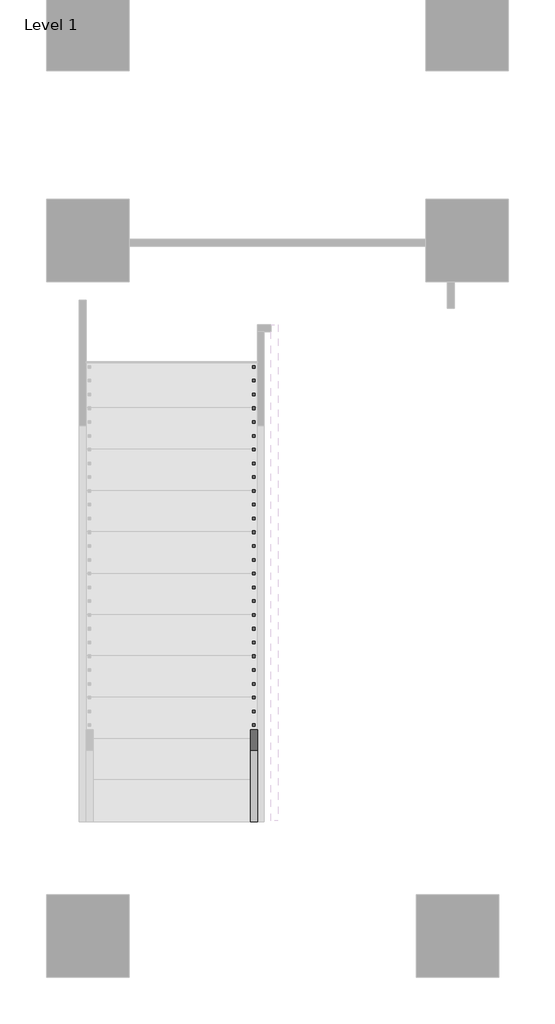
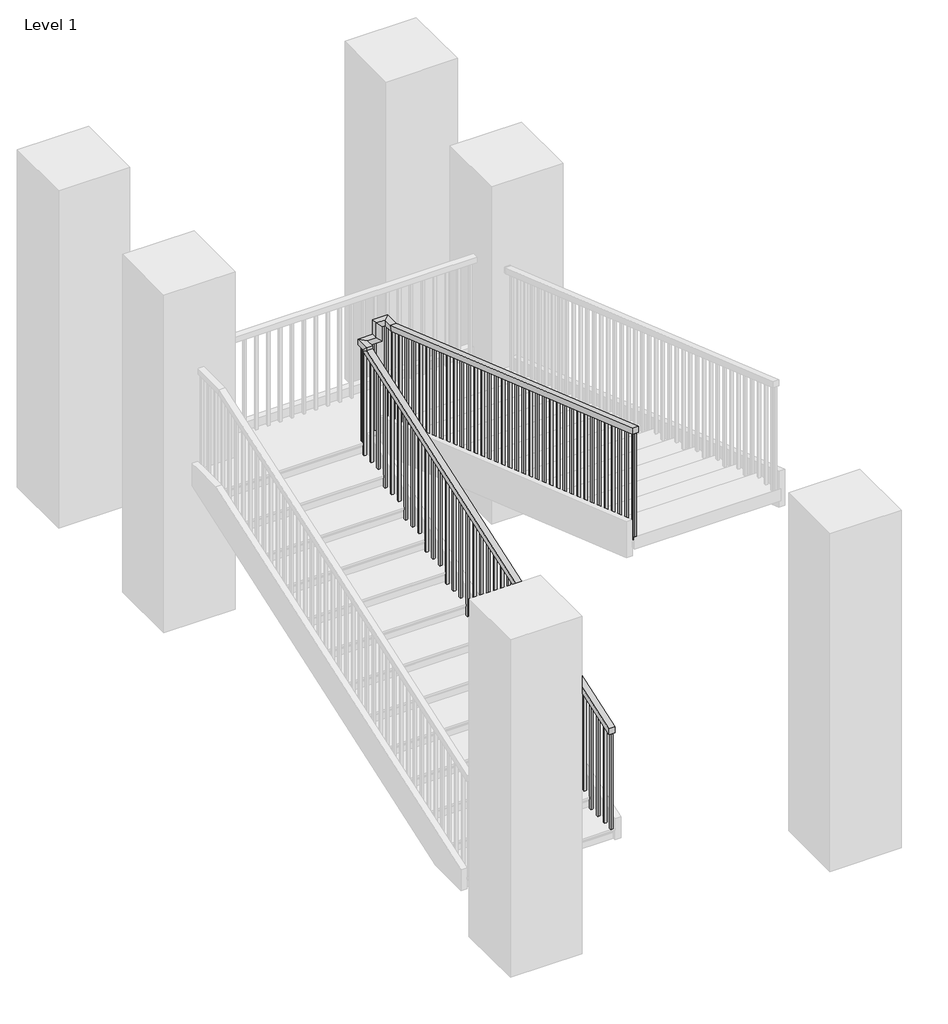
# One storey, part 3 of 6: 1 railing.
"""IFC4 building model written with IfcOpenShell, lengths in millimetres."""

from ifc_helpers import new_model, si_unit, frame, origin, place, context, project, spatial, polyline, outline, extrude, faceted_brep, element, save

model = new_model("IFC4")

# Units and contexts
model_context = context("Model", 3, world=origin())
ifc_project = project(units=[si_unit("LENGTHUNIT", "METRE", prefix="MILLI")], contexts=[model_context])

# Site, building, storey
site = spatial("IfcSite", under=ifc_project)
building = spatial("IfcBuilding", under=site)
storey = spatial("IfcBuildingStorey", under=building, Name="Level 1", Elevation=0.0)

# Railing
placement = place(None, origin())
element("IfcRailing", 1, ObjectType="Handrail - Rectangular", at=placement, inside=storey, context=model_context, shape_type="SolidModel", body=[
    faceted_brep([(-2644.5381751, -9955.5916506, 1019.9076923), (-2644.5381751, -9955.5916506, 966.1602476), (-2593.7381751, -9955.5916506, 966.1602476), (-2593.7381751, -9955.5916506, 1019.9076923), (-2644.5381751, -6367.8416506, 2259.6687908), (-2644.5381751, -6317.0416506, 2223.4754856), (-2593.7381751, -6317.0416506, 2223.4754856), (-2593.7381751, -6367.8416506, 2259.6687908), (-2644.5381751, -6367.8416506, 2286.0), (-2644.5381751, -6317.0416506, 2235.2), (-2593.7381751, -6317.0416506, 2235.2), (-2593.7381751, -6367.8416506, 2286.0), (-2644.5381751, -6240.8416506, 2286.0), (-2644.5381751, -6240.8416506, 2235.2), (-2593.7381751, -6291.6416506, 2235.2), (-2593.7381751, -6291.6416506, 2286.0), (-2517.5381751, -6240.8416506, 2286.0), (-2466.7381751, -6240.8416506, 2235.2), (-2466.7381751, -6291.6416506, 2235.2), (-2517.5381751, -6291.6416506, 2286.0), (-2517.5381751, -6240.8416506, 2417.8846154), (-2466.7381751, -6240.8416506, 2367.0846154), (-2466.7381751, -6291.6416506, 2367.0846154), (-2517.5381751, -6291.6416506, 2417.8846154), (-2390.5381751, -6240.8416506, 2417.8846154), (-2390.5381751, -6240.8416506, 2367.0846154), (-2441.3381751, -6291.6416506, 2367.0846154), (-2441.3381751, -6291.6416506, 2417.8846154), (-2390.5381751, -6367.8416506, 2417.8846154), (-2390.5381751, -6376.3852679, 2367.0846154), (-2441.3381751, -6376.3852679, 2367.0846154), (-2441.3381751, -6367.8416506, 2417.8846154), (-2390.5381751, -9949.2416506, 3657.6), (-2441.3381751, -9949.2416506, 3657.6), (-2441.3381751, -9949.2416506, 3603.842594), (-2390.5381751, -9949.2416506, 3603.842594)], [[[0, 1, 2, 3]], [[1, 0, 4, 5]], [[2, 1, 5, 6]], [[3, 2, 6, 7]], [[0, 3, 7, 4]], [[5, 4, 8, 9]], [[6, 5, 9, 10]], [[7, 6, 10, 11]], [[4, 7, 11, 8]], [[9, 8, 12, 13]], [[10, 9, 13, 14]], [[11, 10, 14, 15]], [[8, 11, 15, 12]], [[13, 12, 16, 17]], [[14, 13, 17, 18]], [[15, 14, 18, 19]], [[12, 15, 19, 16]], [[17, 16, 20, 21]], [[18, 17, 21, 22]], [[19, 18, 22, 23]], [[16, 19, 23, 20]], [[21, 20, 24, 25]], [[22, 21, 25, 26]], [[23, 22, 26, 27]], [[20, 23, 27, 24]], [[25, 24, 28, 29]], [[26, 25, 29, 30]], [[27, 26, 30, 31]], [[24, 27, 31, 28]], [[32, 33, 34, 35]], [[29, 28, 32, 35]], [[30, 29, 35, 34]], [[31, 30, 34, 33]], [[28, 31, 33, 32]]]),
    extrude(outline(polyline([(-9933.3666506, 3598.3474017), (-9914.3166506, 3591.7531709), (-9914.3166506, 2637.6923077), (-9933.3666506, 2637.6923077), (-9933.3666506, 3598.3474017)])), frame((-2425.4631751, 0.0, 0.0), z_axis=(1.0, 0.0, 0.0), x_axis=(0.0, 1.0, 0.0)), (0.0, 0.0, 1.0), 19.05),
    extrude(outline(polyline([(-9831.7666506, 3563.1781709), (-9812.7166506, 3556.5839402), (-9812.7166506, 2637.6923077), (-9831.7666506, 2637.6923077), (-9831.7666506, 3563.1781709)])), frame((-2425.4631751, 0.0, 0.0), z_axis=(1.0, 0.0, 0.0), x_axis=(0.0, 1.0, 0.0)), (0.0, 0.0, 1.0), 19.05),
    extrude(outline(polyline([(-9730.1666506, 3528.0089402), (-9711.1166506, 3521.4147094), (-9711.1166506, 2637.6923077), (-9730.1666506, 2637.6923077), (-9730.1666506, 3528.0089402)])), frame((-2425.4631751, 0.0, 0.0), z_axis=(1.0, 0.0, 0.0), x_axis=(0.0, 1.0, 0.0)), (0.0, 0.0, 1.0), 19.05),
    extrude(outline(polyline([(-9628.5666506, 3492.8397094), (-9609.5166506, 3486.2454786), (-9609.5166506, 2532.1846154), (-9628.5666506, 2532.1846154), (-9628.5666506, 3492.8397094)])), frame((-2425.4631751, 0.0, 0.0), z_axis=(1.0, 0.0, 0.0), x_axis=(0.0, 1.0, 0.0)), (0.0, 0.0, 1.0), 19.05),
    extrude(outline(polyline([(-9526.9666506, 3457.6704786), (-9507.9166506, 3451.0762479), (-9507.9166506, 2532.1846154), (-9526.9666506, 2532.1846154), (-9526.9666506, 3457.6704786)])), frame((-2425.4631751, 0.0, 0.0), z_axis=(1.0, 0.0, 0.0), x_axis=(0.0, 1.0, 0.0)), (0.0, 0.0, 1.0), 19.05),
    extrude(outline(polyline([(-9425.3666506, 3422.5012479), (-9406.3166506, 3415.9070171), (-9406.3166506, 2532.1846154), (-9425.3666506, 2532.1846154), (-9425.3666506, 3422.5012479)])), frame((-2425.4631751, 0.0, 0.0), z_axis=(1.0, 0.0, 0.0), x_axis=(0.0, 1.0, 0.0)), (0.0, 0.0, 1.0), 19.05),
    extrude(outline(polyline([(-9323.7666506, 3387.3320171), (-9304.7166506, 3380.7377863), (-9304.7166506, 2426.6769231), (-9323.7666506, 2426.6769231), (-9323.7666506, 3387.3320171)])), frame((-2425.4631751, 0.0, 0.0), z_axis=(1.0, 0.0, 0.0), x_axis=(0.0, 1.0, 0.0)), (0.0, 0.0, 1.0), 19.05),
    extrude(outline(polyline([(-9222.1666506, 3352.1627863), (-9203.1166506, 3345.5685556), (-9203.1166506, 2426.6769231), (-9222.1666506, 2426.6769231), (-9222.1666506, 3352.1627863)])), frame((-2425.4631751, 0.0, 0.0), z_axis=(1.0, 0.0, 0.0), x_axis=(0.0, 1.0, 0.0)), (0.0, 0.0, 1.0), 19.05),
    extrude(outline(polyline([(-9120.5666506, 3316.9935556), (-9101.5166506, 3310.3993248), (-9101.5166506, 2426.6769231), (-9120.5666506, 2426.6769231), (-9120.5666506, 3316.9935556)])), frame((-2425.4631751, 0.0, 0.0), z_axis=(1.0, 0.0, 0.0), x_axis=(0.0, 1.0, 0.0)), (0.0, 0.0, 1.0), 19.05),
    extrude(outline(polyline([(-9018.9666506, 3281.8243248), (-8999.9166506, 3275.230094), (-8999.9166506, 2321.1692308), (-9018.9666506, 2321.1692308), (-9018.9666506, 3281.8243248)])), frame((-2425.4631751, 0.0, 0.0), z_axis=(1.0, 0.0, 0.0), x_axis=(0.0, 1.0, 0.0)), (0.0, 0.0, 1.0), 19.05),
    extrude(outline(polyline([(-8917.3666506, 3246.655094), (-8898.3166506, 3240.0608632), (-8898.3166506, 2321.1692308), (-8917.3666506, 2321.1692308), (-8917.3666506, 3246.655094)])), frame((-2425.4631751, 0.0, 0.0), z_axis=(1.0, 0.0, 0.0), x_axis=(0.0, 1.0, 0.0)), (0.0, 0.0, 1.0), 19.05),
    extrude(outline(polyline([(-8815.7666506, 3211.4858632), (-8796.7166506, 3204.8916325), (-8796.7166506, 2321.1692308), (-8815.7666506, 2321.1692308), (-8815.7666506, 3211.4858632)])), frame((-2425.4631751, 0.0, 0.0), z_axis=(1.0, 0.0, 0.0), x_axis=(0.0, 1.0, 0.0)), (0.0, 0.0, 1.0), 19.05),
    extrude(outline(polyline([(-8714.1666506, 3176.3166325), (-8695.1166506, 3169.7224017), (-8695.1166506, 2215.6615385), (-8714.1666506, 2215.6615385), (-8714.1666506, 3176.3166325)])), frame((-2425.4631751, 0.0, 0.0), z_axis=(1.0, 0.0, 0.0), x_axis=(0.0, 1.0, 0.0)), (0.0, 0.0, 1.0), 19.05),
    extrude(outline(polyline([(-8612.5666506, 3141.1474017), (-8593.5166506, 3134.5531709), (-8593.5166506, 2215.6615385), (-8612.5666506, 2215.6615385), (-8612.5666506, 3141.1474017)])), frame((-2425.4631751, 0.0, 0.0), z_axis=(1.0, 0.0, 0.0), x_axis=(0.0, 1.0, 0.0)), (0.0, 0.0, 1.0), 19.05),
    extrude(outline(polyline([(-8510.9666506, 3105.9781709), (-8491.9166506, 3099.3839402), (-8491.9166506, 2215.6615385), (-8510.9666506, 2215.6615385), (-8510.9666506, 3105.9781709)])), frame((-2425.4631751, 0.0, 0.0), z_axis=(1.0, 0.0, 0.0), x_axis=(0.0, 1.0, 0.0)), (0.0, 0.0, 1.0), 19.05),
    extrude(outline(polyline([(-8409.3666506, 3070.8089402), (-8390.3166506, 3064.2147094), (-8390.3166506, 2110.1538462), (-8409.3666506, 2110.1538462), (-8409.3666506, 3070.8089402)])), frame((-2425.4631751, 0.0, 0.0), z_axis=(1.0, 0.0, 0.0), x_axis=(0.0, 1.0, 0.0)), (0.0, 0.0, 1.0), 19.05),
    extrude(outline(polyline([(-8307.7666506, 3035.6397094), (-8288.7166506, 3029.0454786), (-8288.7166506, 2110.1538462), (-8307.7666506, 2110.1538462), (-8307.7666506, 3035.6397094)])), frame((-2425.4631751, 0.0, 0.0), z_axis=(1.0, 0.0, 0.0), x_axis=(0.0, 1.0, 0.0)), (0.0, 0.0, 1.0), 19.05),
    extrude(outline(polyline([(-8206.1666506, 3000.4704786), (-8187.1166506, 2993.8762479), (-8187.1166506, 2110.1538462), (-8206.1666506, 2110.1538462), (-8206.1666506, 3000.4704786)])), frame((-2425.4631751, 0.0, 0.0), z_axis=(1.0, 0.0, 0.0), x_axis=(0.0, 1.0, 0.0)), (0.0, 0.0, 1.0), 19.05),
    extrude(outline(polyline([(-8104.5666506, 2965.3012479), (-8085.5166506, 2958.7070171), (-8085.5166506, 2004.6461538), (-8104.5666506, 2004.6461538), (-8104.5666506, 2965.3012479)])), frame((-2425.4631751, 0.0, 0.0), z_axis=(1.0, 0.0, 0.0), x_axis=(0.0, 1.0, 0.0)), (0.0, 0.0, 1.0), 19.05),
    extrude(outline(polyline([(-8002.9666506, 2930.1320171), (-7983.9166506, 2923.5377863), (-7983.9166506, 2004.6461538), (-8002.9666506, 2004.6461538), (-8002.9666506, 2930.1320171)])), frame((-2425.4631751, 0.0, 0.0), z_axis=(1.0, 0.0, 0.0), x_axis=(0.0, 1.0, 0.0)), (0.0, 0.0, 1.0), 19.05),
    extrude(outline(polyline([(-7901.3666506, 2894.9627863), (-7882.3166506, 2888.3685556), (-7882.3166506, 2004.6461538), (-7901.3666506, 2004.6461538), (-7901.3666506, 2894.9627863)])), frame((-2425.4631751, 0.0, 0.0), z_axis=(1.0, 0.0, 0.0), x_axis=(0.0, 1.0, 0.0)), (0.0, 0.0, 1.0), 19.05),
    extrude(outline(polyline([(-7799.7666506, 2859.7935556), (-7780.7166506, 2853.1993248), (-7780.7166506, 1899.1384615), (-7799.7666506, 1899.1384615), (-7799.7666506, 2859.7935556)])), frame((-2425.4631751, 0.0, 0.0), z_axis=(1.0, 0.0, 0.0), x_axis=(0.0, 1.0, 0.0)), (0.0, 0.0, 1.0), 19.05),
    extrude(outline(polyline([(-7698.1666506, 2824.6243248), (-7679.1166506, 2818.030094), (-7679.1166506, 1899.1384615), (-7698.1666506, 1899.1384615), (-7698.1666506, 2824.6243248)])), frame((-2425.4631751, 0.0, 0.0), z_axis=(1.0, 0.0, 0.0), x_axis=(0.0, 1.0, 0.0)), (0.0, 0.0, 1.0), 19.05),
    extrude(outline(polyline([(-7596.5666506, 2789.455094), (-7577.5166506, 2782.8608632), (-7577.5166506, 1899.1384615), (-7596.5666506, 1899.1384615), (-7596.5666506, 2789.455094)])), frame((-2425.4631751, 0.0, 0.0), z_axis=(1.0, 0.0, 0.0), x_axis=(0.0, 1.0, 0.0)), (0.0, 0.0, 1.0), 19.05),
    extrude(outline(polyline([(-7494.9666506, 2754.2858632), (-7475.9166506, 2747.6916325), (-7475.9166506, 1793.6307692), (-7494.9666506, 1793.6307692), (-7494.9666506, 2754.2858632)])), frame((-2425.4631751, 0.0, 0.0), z_axis=(1.0, 0.0, 0.0), x_axis=(0.0, 1.0, 0.0)), (0.0, 0.0, 1.0), 19.05),
    extrude(outline(polyline([(-7393.3666506, 2719.1166325), (-7374.3166506, 2712.5224017), (-7374.3166506, 1793.6307692), (-7393.3666506, 1793.6307692), (-7393.3666506, 2719.1166325)])), frame((-2425.4631751, 0.0, 0.0), z_axis=(1.0, 0.0, 0.0), x_axis=(0.0, 1.0, 0.0)), (0.0, 0.0, 1.0), 19.05),
    extrude(outline(polyline([(-7291.7666506, 2683.9474017), (-7272.7166506, 2677.3531709), (-7272.7166506, 1793.6307692), (-7291.7666506, 1793.6307692), (-7291.7666506, 2683.9474017)])), frame((-2425.4631751, 0.0, 0.0), z_axis=(1.0, 0.0, 0.0), x_axis=(0.0, 1.0, 0.0)), (0.0, 0.0, 1.0), 19.05),
    extrude(outline(polyline([(-7190.1666506, 2648.7781709), (-7171.1166506, 2642.1839402), (-7171.1166506, 1688.1230769), (-7190.1666506, 1688.1230769), (-7190.1666506, 2648.7781709)])), frame((-2425.4631751, 0.0, 0.0), z_axis=(1.0, 0.0, 0.0), x_axis=(0.0, 1.0, 0.0)), (0.0, 0.0, 1.0), 19.05),
    extrude(outline(polyline([(-7088.5666506, 2613.6089402), (-7069.5166506, 2607.0147094), (-7069.5166506, 1688.1230769), (-7088.5666506, 1688.1230769), (-7088.5666506, 2613.6089402)])), frame((-2425.4631751, 0.0, 0.0), z_axis=(1.0, 0.0, 0.0), x_axis=(0.0, 1.0, 0.0)), (0.0, 0.0, 1.0), 19.05),
    extrude(outline(polyline([(-6986.9666506, 2578.4397094), (-6967.9166506, 2571.8454786), (-6967.9166506, 1688.1230769), (-6986.9666506, 1688.1230769), (-6986.9666506, 2578.4397094)])), frame((-2425.4631751, 0.0, 0.0), z_axis=(1.0, 0.0, 0.0), x_axis=(0.0, 1.0, 0.0)), (0.0, 0.0, 1.0), 19.05),
    extrude(outline(polyline([(-6885.3666506, 2543.2704786), (-6866.3166506, 2536.6762479), (-6866.3166506, 1582.6153846), (-6885.3666506, 1582.6153846), (-6885.3666506, 2543.2704786)])), frame((-2425.4631751, 0.0, 0.0), z_axis=(1.0, 0.0, 0.0), x_axis=(0.0, 1.0, 0.0)), (0.0, 0.0, 1.0), 19.05),
    extrude(outline(polyline([(-6783.7666506, 2508.1012479), (-6764.7166506, 2501.5070171), (-6764.7166506, 1582.6153846), (-6783.7666506, 1582.6153846), (-6783.7666506, 2508.1012479)])), frame((-2425.4631751, 0.0, 0.0), z_axis=(1.0, 0.0, 0.0), x_axis=(0.0, 1.0, 0.0)), (0.0, 0.0, 1.0), 19.05),
    extrude(outline(polyline([(-6682.1666506, 2472.9320171), (-6663.1166506, 2466.3377863), (-6663.1166506, 1582.6153846), (-6682.1666506, 1582.6153846), (-6682.1666506, 2472.9320171)])), frame((-2425.4631751, 0.0, 0.0), z_axis=(1.0, 0.0, 0.0), x_axis=(0.0, 1.0, 0.0)), (0.0, 0.0, 1.0), 19.05),
    extrude(outline(polyline([(-6580.5666506, 2437.7627863), (-6561.5166506, 2431.1685556), (-6561.5166506, 1477.1076923), (-6580.5666506, 1477.1076923), (-6580.5666506, 2437.7627863)])), frame((-2425.4631751, 0.0, 0.0), z_axis=(1.0, 0.0, 0.0), x_axis=(0.0, 1.0, 0.0)), (0.0, 0.0, 1.0), 19.05),
    extrude(outline(polyline([(-6478.9666506, 2402.5935556), (-6459.9166506, 2395.9993248), (-6459.9166506, 1477.1076923), (-6478.9666506, 1477.1076923), (-6478.9666506, 2402.5935556)])), frame((-2425.4631751, 0.0, 0.0), z_axis=(1.0, 0.0, 0.0), x_axis=(0.0, 1.0, 0.0)), (0.0, 0.0, 1.0), 19.05),
    extrude(outline(polyline([(-6377.3666506, 2367.4243248), (-6358.3166506, 2360.830094), (-6358.3166506, 1477.1076923), (-6377.3666506, 1477.1076923), (-6377.3666506, 2367.4243248)])), frame((-2425.4631751, 0.0, 0.0), z_axis=(1.0, 0.0, 0.0), x_axis=(0.0, 1.0, 0.0)), (0.0, 0.0, 1.0), 19.05),
    extrude(outline(polyline([(-2527.0631751, -6275.7666506), (-2527.0631751, -6256.7166506), (-2508.0131751, -6256.7166506), (-2508.0131751, -6275.7666506), (-2527.0631751, -6275.7666506)])), frame((0.0, 0.0, 1371.6), z_axis=(0.0, 0.0, 1.0), x_axis=(1.0, 0.0, 0.0)), (0.0, 0.0, 1.0), 863.6),
    extrude(outline(polyline([(-2609.6131751, -6307.5166506), (-2628.6631751, -6307.5166506), (-2628.6631751, -6288.4666506), (-2609.6131751, -6288.4666506), (-2609.6131751, -6307.5166506)])), frame((0.0, 0.0, 1266.0923077), z_axis=(0.0, 0.0, 1.0), x_axis=(1.0, 0.0, 0.0)), (0.0, 0.0, 1.0), 969.1076923),
    extrude(outline(polyline([(-6409.1166506, 2191.6586078), (-6390.0666506, 2198.2414101), (-6390.0666506, 1266.0923077), (-6409.1166506, 1266.0923077), (-6409.1166506, 2191.6586078)])), frame((-2628.6631751, 0.0, 0.0), z_axis=(1.0, 0.0, 0.0), x_axis=(0.0, 1.0, 0.0)), (0.0, 0.0, 1.0), 19.05),
    extrude(outline(polyline([(-6510.7166506, 2156.5503289), (-6491.6666506, 2163.1331312), (-6491.6666506, 1266.0923077), (-6510.7166506, 1266.0923077), (-6510.7166506, 2156.5503289)])), frame((-2628.6631751, 0.0, 0.0), z_axis=(1.0, 0.0, 0.0), x_axis=(0.0, 1.0, 0.0)), (0.0, 0.0, 1.0), 19.05),
    extrude(outline(polyline([(-6612.3166506, 2121.44205), (-6593.2666506, 2128.0248523), (-6593.2666506, 1160.5846154), (-6612.3166506, 1160.5846154), (-6612.3166506, 2121.44205)])), frame((-2628.6631751, 0.0, 0.0), z_axis=(1.0, 0.0, 0.0), x_axis=(0.0, 1.0, 0.0)), (0.0, 0.0, 1.0), 19.05),
    extrude(outline(polyline([(-6713.9166506, 2086.3337711), (-6694.8666506, 2092.9165734), (-6694.8666506, 1160.5846154), (-6713.9166506, 1160.5846154), (-6713.9166506, 2086.3337711)])), frame((-2628.6631751, 0.0, 0.0), z_axis=(1.0, 0.0, 0.0), x_axis=(0.0, 1.0, 0.0)), (0.0, 0.0, 1.0), 19.05),
    extrude(outline(polyline([(-6815.5166506, 2051.2254922), (-6796.4666506, 2057.8082945), (-6796.4666506, 1160.5846154), (-6815.5166506, 1160.5846154), (-6815.5166506, 2051.2254922)])), frame((-2628.6631751, 0.0, 0.0), z_axis=(1.0, 0.0, 0.0), x_axis=(0.0, 1.0, 0.0)), (0.0, 0.0, 1.0), 19.05),
    extrude(outline(polyline([(-6917.1166506, 2016.1172133), (-6898.0666506, 2022.7000156), (-6898.0666506, 1055.0769231), (-6917.1166506, 1055.0769231), (-6917.1166506, 2016.1172133)])), frame((-2628.6631751, 0.0, 0.0), z_axis=(1.0, 0.0, 0.0), x_axis=(0.0, 1.0, 0.0)), (0.0, 0.0, 1.0), 19.05),
    extrude(outline(polyline([(-7018.7166506, 1981.0089344), (-6999.6666506, 1987.5917367), (-6999.6666506, 1055.0769231), (-7018.7166506, 1055.0769231), (-7018.7166506, 1981.0089344)])), frame((-2628.6631751, 0.0, 0.0), z_axis=(1.0, 0.0, 0.0), x_axis=(0.0, 1.0, 0.0)), (0.0, 0.0, 1.0), 19.05),
    extrude(outline(polyline([(-7120.3166506, 1945.9006556), (-7101.2666506, 1952.4834578), (-7101.2666506, 1055.0769231), (-7120.3166506, 1055.0769231), (-7120.3166506, 1945.9006556)])), frame((-2628.6631751, 0.0, 0.0), z_axis=(1.0, 0.0, 0.0), x_axis=(0.0, 1.0, 0.0)), (0.0, 0.0, 1.0), 19.05),
    extrude(outline(polyline([(-7221.9166506, 1910.7923767), (-7202.8666506, 1917.375179), (-7202.8666506, 949.5692308), (-7221.9166506, 949.5692308), (-7221.9166506, 1910.7923767)])), frame((-2628.6631751, 0.0, 0.0), z_axis=(1.0, 0.0, 0.0), x_axis=(0.0, 1.0, 0.0)), (0.0, 0.0, 1.0), 19.05),
    extrude(outline(polyline([(-7323.5166506, 1875.6840978), (-7304.4666506, 1882.2669001), (-7304.4666506, 949.5692308), (-7323.5166506, 949.5692308), (-7323.5166506, 1875.6840978)])), frame((-2628.6631751, 0.0, 0.0), z_axis=(1.0, 0.0, 0.0), x_axis=(0.0, 1.0, 0.0)), (0.0, 0.0, 1.0), 19.05),
    extrude(outline(polyline([(-7425.1166506, 1840.5758189), (-7406.0666506, 1847.1586212), (-7406.0666506, 949.5692308), (-7425.1166506, 949.5692308), (-7425.1166506, 1840.5758189)])), frame((-2628.6631751, 0.0, 0.0), z_axis=(1.0, 0.0, 0.0), x_axis=(0.0, 1.0, 0.0)), (0.0, 0.0, 1.0), 19.05),
    extrude(outline(polyline([(-7526.7166506, 1805.46754), (-7507.6666506, 1812.0503423), (-7507.6666506, 844.0615385), (-7526.7166506, 844.0615385), (-7526.7166506, 1805.46754)])), frame((-2628.6631751, 0.0, 0.0), z_axis=(1.0, 0.0, 0.0), x_axis=(0.0, 1.0, 0.0)), (0.0, 0.0, 1.0), 19.05),
    extrude(outline(polyline([(-7628.3166506, 1770.3592611), (-7609.2666506, 1776.9420634), (-7609.2666506, 844.0615385), (-7628.3166506, 844.0615385), (-7628.3166506, 1770.3592611)])), frame((-2628.6631751, 0.0, 0.0), z_axis=(1.0, 0.0, 0.0), x_axis=(0.0, 1.0, 0.0)), (0.0, 0.0, 1.0), 19.05),
    extrude(outline(polyline([(-7729.9166506, 1735.2509822), (-7710.8666506, 1741.8337845), (-7710.8666506, 844.0615385), (-7729.9166506, 844.0615385), (-7729.9166506, 1735.2509822)])), frame((-2628.6631751, 0.0, 0.0), z_axis=(1.0, 0.0, 0.0), x_axis=(0.0, 1.0, 0.0)), (0.0, 0.0, 1.0), 19.05),
    extrude(outline(polyline([(-7831.5166506, 1700.1427033), (-7812.4666506, 1706.7255056), (-7812.4666506, 738.5538462), (-7831.5166506, 738.5538462), (-7831.5166506, 1700.1427033)])), frame((-2628.6631751, 0.0, 0.0), z_axis=(1.0, 0.0, 0.0), x_axis=(0.0, 1.0, 0.0)), (0.0, 0.0, 1.0), 19.05),
    extrude(outline(polyline([(-7933.1166506, 1665.0344244), (-7914.0666506, 1671.6172267), (-7914.0666506, 738.5538462), (-7933.1166506, 738.5538462), (-7933.1166506, 1665.0344244)])), frame((-2628.6631751, 0.0, 0.0), z_axis=(1.0, 0.0, 0.0), x_axis=(0.0, 1.0, 0.0)), (0.0, 0.0, 1.0), 19.05),
    extrude(outline(polyline([(-8034.7166506, 1629.9261455), (-8015.6666506, 1636.5089478), (-8015.6666506, 738.5538462), (-8034.7166506, 738.5538462), (-8034.7166506, 1629.9261455)])), frame((-2628.6631751, 0.0, 0.0), z_axis=(1.0, 0.0, 0.0), x_axis=(0.0, 1.0, 0.0)), (0.0, 0.0, 1.0), 19.05),
    extrude(outline(polyline([(-8136.3166506, 1594.8178666), (-8117.2666506, 1601.4006689), (-8117.2666506, 633.0461538), (-8136.3166506, 633.0461538), (-8136.3166506, 1594.8178666)])), frame((-2628.6631751, 0.0, 0.0), z_axis=(1.0, 0.0, 0.0), x_axis=(0.0, 1.0, 0.0)), (0.0, 0.0, 1.0), 19.05),
    extrude(outline(polyline([(-8237.9166506, 1559.7095877), (-8218.8666506, 1566.29239), (-8218.8666506, 633.0461538), (-8237.9166506, 633.0461538), (-8237.9166506, 1559.7095877)])), frame((-2628.6631751, 0.0, 0.0), z_axis=(1.0, 0.0, 0.0), x_axis=(0.0, 1.0, 0.0)), (0.0, 0.0, 1.0), 19.05),
    extrude(outline(polyline([(-8339.5166506, 1524.6013088), (-8320.4666506, 1531.1841111), (-8320.4666506, 633.0461538), (-8339.5166506, 633.0461538), (-8339.5166506, 1524.6013088)])), frame((-2628.6631751, 0.0, 0.0), z_axis=(1.0, 0.0, 0.0), x_axis=(0.0, 1.0, 0.0)), (0.0, 0.0, 1.0), 19.05),
    extrude(outline(polyline([(-8441.1166506, 1489.4930299), (-8422.0666506, 1496.0758322), (-8422.0666506, 527.5384615), (-8441.1166506, 527.5384615), (-8441.1166506, 1489.4930299)])), frame((-2628.6631751, 0.0, 0.0), z_axis=(1.0, 0.0, 0.0), x_axis=(0.0, 1.0, 0.0)), (0.0, 0.0, 1.0), 19.05),
    extrude(outline(polyline([(-8542.7166506, 1454.384751), (-8523.6666506, 1460.9675533), (-8523.6666506, 527.5384615), (-8542.7166506, 527.5384615), (-8542.7166506, 1454.384751)])), frame((-2628.6631751, 0.0, 0.0), z_axis=(1.0, 0.0, 0.0), x_axis=(0.0, 1.0, 0.0)), (0.0, 0.0, 1.0), 19.05),
    extrude(outline(polyline([(-8644.3166506, 1419.2764721), (-8625.2666506, 1425.8592744), (-8625.2666506, 527.5384615), (-8644.3166506, 527.5384615), (-8644.3166506, 1419.2764721)])), frame((-2628.6631751, 0.0, 0.0), z_axis=(1.0, 0.0, 0.0), x_axis=(0.0, 1.0, 0.0)), (0.0, 0.0, 1.0), 19.05),
    extrude(outline(polyline([(-8745.9166506, 1384.1681932), (-8726.8666506, 1390.7509955), (-8726.8666506, 422.0307692), (-8745.9166506, 422.0307692), (-8745.9166506, 1384.1681932)])), frame((-2628.6631751, 0.0, 0.0), z_axis=(1.0, 0.0, 0.0), x_axis=(0.0, 1.0, 0.0)), (0.0, 0.0, 1.0), 19.05),
    extrude(outline(polyline([(-8847.5166506, 1349.0599143), (-8828.4666506, 1355.6427166), (-8828.4666506, 422.0307692), (-8847.5166506, 422.0307692), (-8847.5166506, 1349.0599143)])), frame((-2628.6631751, 0.0, 0.0), z_axis=(1.0, 0.0, 0.0), x_axis=(0.0, 1.0, 0.0)), (0.0, 0.0, 1.0), 19.05),
    extrude(outline(polyline([(-8949.1166506, 1313.9516354), (-8930.0666506, 1320.5344377), (-8930.0666506, 422.0307692), (-8949.1166506, 422.0307692), (-8949.1166506, 1313.9516354)])), frame((-2628.6631751, 0.0, 0.0), z_axis=(1.0, 0.0, 0.0), x_axis=(0.0, 1.0, 0.0)), (0.0, 0.0, 1.0), 19.05),
    extrude(outline(polyline([(-9050.7166506, 1278.8433565), (-9031.6666506, 1285.4261588), (-9031.6666506, 316.5230769), (-9050.7166506, 316.5230769), (-9050.7166506, 1278.8433565)])), frame((-2628.6631751, 0.0, 0.0), z_axis=(1.0, 0.0, 0.0), x_axis=(0.0, 1.0, 0.0)), (0.0, 0.0, 1.0), 19.05),
    extrude(outline(polyline([(-9152.3166506, 1243.7350776), (-9133.2666506, 1250.3178799), (-9133.2666506, 316.5230769), (-9152.3166506, 316.5230769), (-9152.3166506, 1243.7350776)])), frame((-2628.6631751, 0.0, 0.0), z_axis=(1.0, 0.0, 0.0), x_axis=(0.0, 1.0, 0.0)), (0.0, 0.0, 1.0), 19.05),
    extrude(outline(polyline([(-9253.9166506, 1208.6267987), (-9234.8666506, 1215.209601), (-9234.8666506, 316.5230769), (-9253.9166506, 316.5230769), (-9253.9166506, 1208.6267987)])), frame((-2628.6631751, 0.0, 0.0), z_axis=(1.0, 0.0, 0.0), x_axis=(0.0, 1.0, 0.0)), (0.0, 0.0, 1.0), 19.05),
    extrude(outline(polyline([(-9355.5166506, 1173.5185198), (-9336.4666506, 1180.1013221), (-9336.4666506, 211.0153846), (-9355.5166506, 211.0153846), (-9355.5166506, 1173.5185198)])), frame((-2628.6631751, 0.0, 0.0), z_axis=(1.0, 0.0, 0.0), x_axis=(0.0, 1.0, 0.0)), (0.0, 0.0, 1.0), 19.05),
    extrude(outline(polyline([(-9457.1166506, 1138.4102409), (-9438.0666506, 1144.9930432), (-9438.0666506, 211.0153846), (-9457.1166506, 211.0153846), (-9457.1166506, 1138.4102409)])), frame((-2628.6631751, 0.0, 0.0), z_axis=(1.0, 0.0, 0.0), x_axis=(0.0, 1.0, 0.0)), (0.0, 0.0, 1.0), 19.05),
    extrude(outline(polyline([(-9558.7166506, 1103.301962), (-9539.6666506, 1109.8847643), (-9539.6666506, 211.0153846), (-9558.7166506, 211.0153846), (-9558.7166506, 1103.301962)])), frame((-2628.6631751, 0.0, 0.0), z_axis=(1.0, 0.0, 0.0), x_axis=(0.0, 1.0, 0.0)), (0.0, 0.0, 1.0), 19.05),
    extrude(outline(polyline([(-9660.3166506, 1068.1936831), (-9641.2666506, 1074.7764854), (-9641.2666506, 105.5076923), (-9660.3166506, 105.5076923), (-9660.3166506, 1068.1936831)])), frame((-2628.6631751, 0.0, 0.0), z_axis=(1.0, 0.0, 0.0), x_axis=(0.0, 1.0, 0.0)), (0.0, 0.0, 1.0), 19.05),
    extrude(outline(polyline([(-9761.9166506, 1033.0854043), (-9742.8666506, 1039.6682065), (-9742.8666506, 105.5076923), (-9761.9166506, 105.5076923), (-9761.9166506, 1033.0854043)])), frame((-2628.6631751, 0.0, 0.0), z_axis=(1.0, 0.0, 0.0), x_axis=(0.0, 1.0, 0.0)), (0.0, 0.0, 1.0), 19.05),
    extrude(outline(polyline([(-9863.5166506, 997.9771254), (-9844.4666506, 1004.5599277), (-9844.4666506, 105.5076923), (-9863.5166506, 105.5076923), (-9863.5166506, 997.9771254)])), frame((-2628.6631751, 0.0, 0.0), z_axis=(1.0, 0.0, 0.0), x_axis=(0.0, 1.0, 0.0)), (0.0, 0.0, 1.0), 19.05),
    extrude(outline(polyline([(-2425.4631751, -6275.7666506), (-2425.4631751, -6256.7166506), (-2406.4131751, -6256.7166506), (-2406.4131751, -6275.7666506), (-2425.4631751, -6275.7666506)])), frame((0.0, 0.0, 1371.6), z_axis=(0.0, 0.0, 1.0), x_axis=(1.0, 0.0, 0.0)), (0.0, 0.0, 1.0), 995.4846154),
    extrude(outline(polyline([(-2609.6131751, -6275.7666506), (-2628.6631751, -6275.7666506), (-2628.6631751, -6256.7166506), (-2609.6131751, -6256.7166506), (-2609.6131751, -6275.7666506)])), frame((0.0, 0.0, 1371.6), z_axis=(0.0, 0.0, 1.0), x_axis=(1.0, 0.0, 0.0)), (0.0, 0.0, 1.0), 863.6),
    extrude(outline(polyline([(-9949.2416506, 3603.842594), (-9930.1916506, 3597.2483632), (-9930.1916506, 2637.6923077), (-9949.2416506, 2637.6923077), (-9949.2416506, 3603.842594)])), frame((-2425.4631751, 0.0, 0.0), z_axis=(1.0, 0.0, 0.0), x_axis=(0.0, 1.0, 0.0)), (0.0, 0.0, 1.0), 19.05),
    extrude(outline(polyline([(-9955.5916506, 966.1602476), (-9936.5416506, 972.7430499), (-9936.5416506, 105.5076923), (-9955.5916506, 105.5076923), (-9955.5916506, 966.1602476)])), frame((-2628.6631751, 0.0, 0.0), z_axis=(1.0, 0.0, 0.0), x_axis=(0.0, 1.0, 0.0)), (0.0, 0.0, 1.0), 19.05),
])

save(model, "model.ifc")

# Revit data of these elements
# Type "Handrail - Rectangular"
#   Assembly Code = "C2010400"
#   built-in parameter 1008612 = 0.0416667 (stored number, unit not read)
#   built-in parameter 1008611 = 0.0416667 (stored number, unit not read)
#   built-in parameter 1008609 = 0.333333 (stored number, unit not read)
#   built-in parameter 1008604 = 0.166667 (stored number, unit not read)
#   built-in parameter 1008603 = 0.166667 (stored number, unit not read)
#   Railing Height = 3' - 0"
#   built-in parameter 1008630 = 2
#   built-in parameter 1008610 = 2
#   built-in parameter 1008618 = Baluster - Square : 3/4"
# Element 1 (IfcRailing, "Handrail - Rectangular")
#   Phase Created = New Construction
